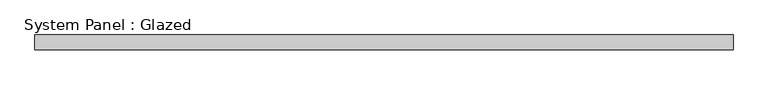
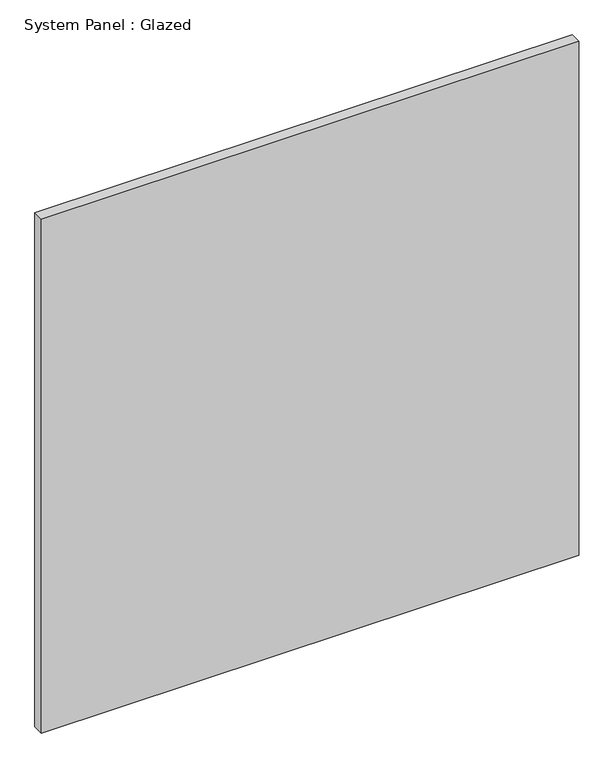
"""IFC4 building model written with IfcOpenShell, lengths in millimetres: plate geometry, System Panel : Glazed."""

from ifc_helpers import new_model, si_unit, origin, origin_with_axes, place, context, project, spatial, polyline, outline, extrude, source, transform, mapped, element, save


def system_panel_glazed_0f25c23b(model_context):
    return source(origin(), model_context, "Body", "SweptSolid", [
        extrude(outline(polyline([(603.25, 19.05), (-603.25, 19.05), (-603.25, 44.45), (603.25, 44.45), (603.25, 19.05)])), origin_with_axes(), (0.0, 0.0, 1.0), 1219.2),
    ])


if __name__ == "__main__":
    model = new_model("IFC4")
    model_context = context("Model", 3, world=origin())
    ifc_project = project(units=[si_unit("LENGTHUNIT", "METRE", prefix="MILLI")], contexts=[model_context])
    site = spatial("IfcSite", under=ifc_project)
    building = spatial("IfcBuilding", under=site)
    placement = place(None, origin())
    system_panel_glazed_shape = system_panel_glazed_0f25c23b(model_context)
    element("IfcPlate", 1, ObjectType="System Panel : Glazed", at=placement, inside=building, context=model_context, shape_type="MappedRepresentation", body=[
        mapped(system_panel_glazed_shape, transform((0.0, 0.0, 0.0), x_axis=(1.0, 0.0, 0.0), y_axis=(0.0, 1.0, 0.0), z_axis=(0.0, 0.0, 1.0))),
    ])
    save(model, "model.ifc")

# Revit data of these elements
# Type "System Panel : Glazed"
#   Construction Type Id = "GSP4R"
#   Analytic Construction = "1/8 in Pilkington single glazing"
#   Visual Light Transmittance = 0.9
#   Solar Heat Gain Coefficient = 0.86
#   Heat Transfer Coefficient (U) = 1.18115 BTU/(h·ft²·°F)
# Element 1 (IfcPlate, "System Panel : Glazed")
#   Materials on its faces: "Glass"
# Materials
#   "Glass": class "Glass", colour RGB 0 128 192, transparency 0.75, Description = "Soda Lime Glass", Cost = 0
